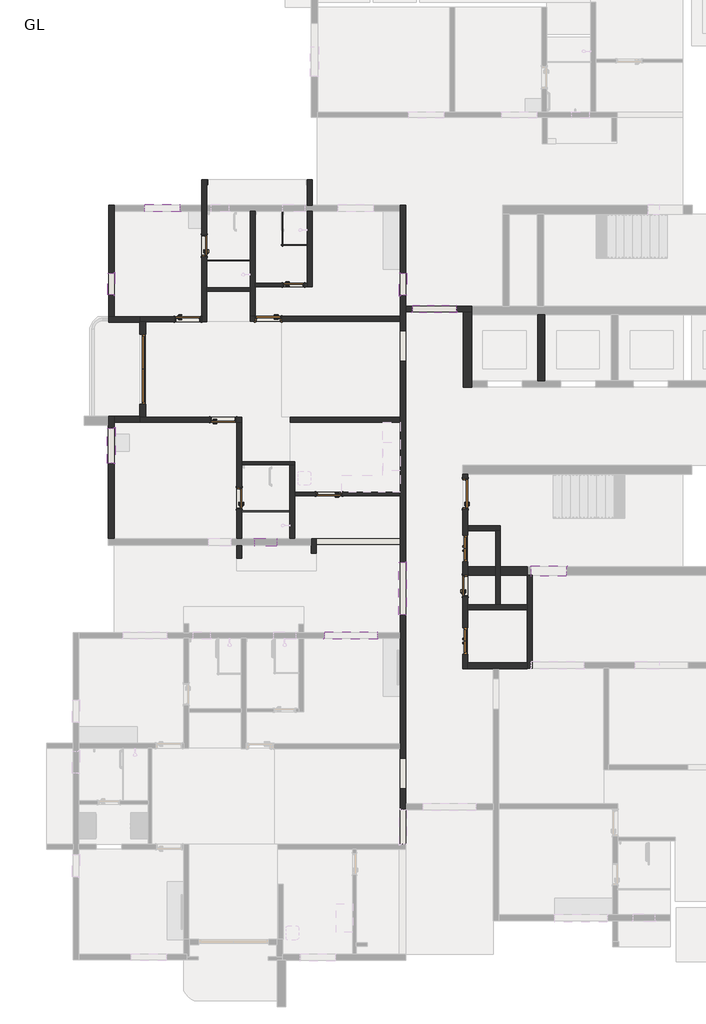
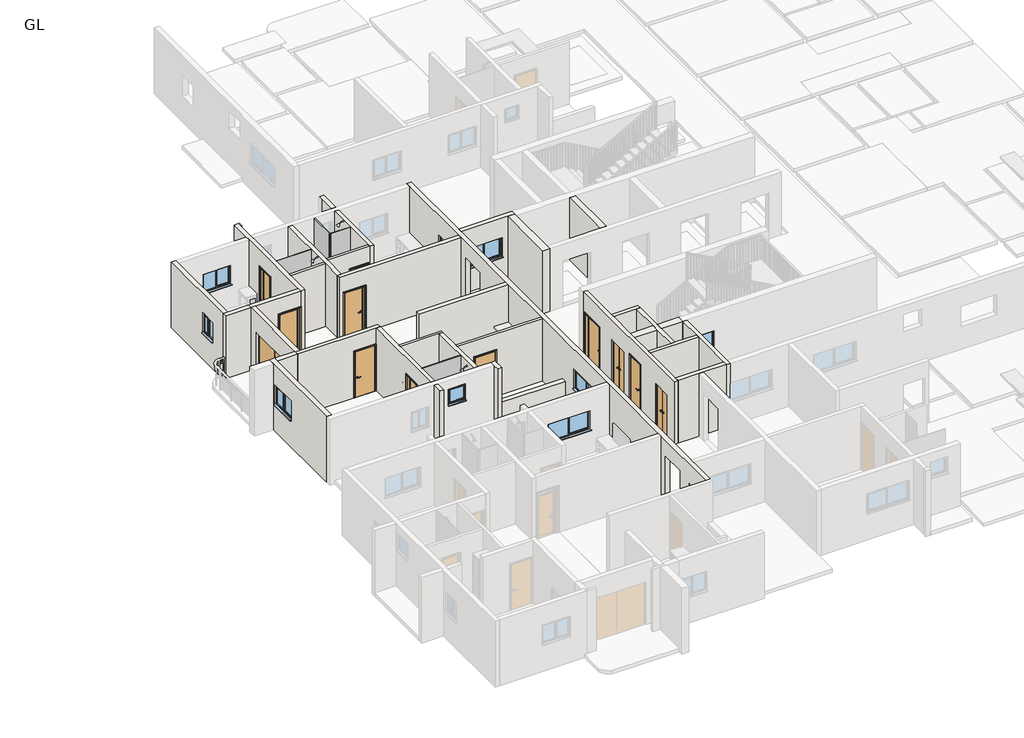
# One storey, part 2 of 14: 32 walls, 12 doors, 9 windows, 4 plates.
# Revit data of these elements (continued)
# Type "Windows_Dbl_Plain : 2.5'" (continued)
#   Analytic Construction = "1/8 in Pilkington single glazing"
#   Wrap Layers (Ext) from Ext = 0.336286 ft
#   Wrap Layers (Int) from Ext = 0.582349 ft
#   Window Board Projection = 0.082021 ft
#   Window Board Extension = 0.082021 ft
#   Visual Light Transmittance = 0.9
#   Solar Heat Gain Coefficient = 0.78
#   Rough Width = 2.5 ft
#   Rough Height = 2.985564 ft
#   Height = 2.985564 ft
#   Width = 2.5 ft
#   Heat Transfer Coefficient (U) = 3.6886 W/(m²·K)
#   Glazing Thickness = 0.07874 ft
#   FrameOffset - External = 0.164042 ft
#   Frame Depth = 0.213255 ft
#   Default Head Height = 6.922572 ft
#   Cill Depth = 0.287073 ft
#   Cavity Closer Width = 0.164042 ft
#   Cavity Closer Offset from Ext = 0.336286 ft
#   Cavity Closer Depth = 0.278871 ft
#   Vis - Cavity Closers = yes
#   Define Thermal Properties by = 1
#   Material Trim = Window Frame
#   Material Glass = Glass
#   Material Frame = Window Frame
#   Wall Closure = (empty or 0)
# Type "Windows_Dbl_Plain : 4'"
#   Type Mark = "56"
#   Operation = "DoublePanelVertical"
#   Construction Type Id = "GSP4R"
#   Manufacturer = "Revit"
#   Keynote = "L10"
#   Analytic Construction = "1/8 in Pilkington single glazing"
#   Wrap Layers (Ext) from Ext = 0.336286 ft
#   Wrap Layers (Int) from Ext = 0.582349 ft
#   Window Board Projection = 0.082021 ft
#   Window Board Extension = 0.082021 ft
#   Visual Light Transmittance = 0.9
#   Solar Heat Gain Coefficient = 0.78
#   Rough Width = 4.0 ft
#   Rough Height = 2.985564 ft
#   Height = 2.985564 ft
#   Width = 4.0 ft
#   Heat Transfer Coefficient (U) = 3.6886 W/(m²·K)
#   Glazing Thickness = 0.07874 ft
#   FrameOffset - External = 0.164042 ft
#   Frame Depth = 0.213255 ft
#   Default Head Height = 6.922572 ft
#   Cill Depth = 0.287073 ft
#   Cavity Closer Width = 0.164042 ft
#   Cavity Closer Offset from Ext = 0.336286 ft
#   Cavity Closer Depth = 0.278871 ft
#   Vis - Cavity Closers = yes
#   Define Thermal Properties by = 1
#   Material Trim = Window Frame
#   Material Glass = Glass
#   Material Frame = Window Frame
#   Wall Closure = (empty or 0)
# Type "Windows_Dbl_Plain : 5'"
#   Type Mark = "58"
#   Operation = "DoublePanelVertical"
#   Construction Type Id = "GSP4R"
#   Manufacturer = "Revit"
#   Keynote = "L10"
#   Analytic Construction = "1/8 in Pilkington single glazing"
#   Wrap Layers (Ext) from Ext = 0.336286 ft
#   Wrap Layers (Int) from Ext = 0.582349 ft
#   Window Board Projection = 0.082021 ft
#   Window Board Extension = 0.082021 ft
#   Visual Light Transmittance = 0.9
#   Solar Heat Gain Coefficient = 0.78
#   Rough Width = 5.0 ft
#   Rough Height = 2.985564 ft
#   Height = 2.985564 ft
#   Width = 5.0 ft
#   Heat Transfer Coefficient (U) = 3.6886 W/(m²·K)
#   Glazing Thickness = 0.07874 ft
#   FrameOffset - External = 0.164042 ft
#   Frame Depth = 0.213255 ft
#   Default Head Height = 6.922572 ft
#   Cill Depth = 0.287073 ft
#   Cavity Closer Width = 0.164042 ft
#   Cavity Closer Offset from Ext = 0.336286 ft
#   Cavity Closer Depth = 0.278871 ft
#   Vis - Cavity Closers = yes
#   Define Thermal Properties by = 1
#   Material Trim = Window Frame
#   Material Glass = Glass
#   Material Frame = Window Frame
#   Wall Closure = (empty or 0)
# Type "Windows_Dbl_Plain : 6'"
#   Type Mark = "62"
#   Operation = "DoublePanelVertical"
#   Construction Type Id = "GSP4R"
#   Manufacturer = "Revit"
#   Keynote = "L10"
#   Analytic Construction = "1/8 in Pilkington single glazing"
#   Wrap Layers (Ext) from Ext = 0.336286 ft
#   Wrap Layers (Int) from Ext = 0.582349 ft
#   Window Board Projection = 0.082021 ft
#   Window Board Extension = 0.082021 ft
#   Visual Light Transmittance = 0.9
#   Solar Heat Gain Coefficient = 0.78
#   Rough Width = 6.0 ft
#   Rough Height = 2.985564 ft
#   Height = 2.985564 ft
#   Width = 6.0 ft
#   Heat Transfer Coefficient (U) = 3.6886 W/(m²·K)
#   Glazing Thickness = 0.07874 ft
#   FrameOffset - External = 0.164042 ft
#   Frame Depth = 0.213255 ft
#   Default Head Height = 6.922572 ft
#   Cill Depth = 0.287073 ft
#   Cavity Closer Width = 0.164042 ft
#   Cavity Closer Offset from Ext = 0.336286 ft
#   Cavity Closer Depth = 0.278871 ft
#   Vis - Cavity Closers = yes
#   Define Thermal Properties by = 1
#   Material Trim = Window Frame
#   Material Glass = Glass
#   Material Frame = Window Frame
#   Wall Closure = (empty or 0)
# Type "Windows_Sgl_Plain : 2.5'"
#   Type Mark = "61"
#   Operation = "SinglePanel"
#   Construction Type Id = "SGL"
#   Manufacturer = "Revit"
#   Keynote = "L10"
#   Analytic Construction = "Large single-glazed windows"
#   Wrap Layers (Ext) from Ext = 0.336286 ft
#   Wrap Layers (Int) from Ext = 0.582349 ft
#   Window Board Projection = 0.082021 ft
#   Window Board Extension = 0.082021 ft
#   Visual Light Transmittance = 0.9
#   Solar Heat Gain Coefficient = 0.86
#   Rough Width = 2.5 ft
#   Rough Height = 2.5 ft
#   Height = 2.5 ft
#   Width = 2.5 ft
#   Heat Transfer Coefficient (U) = 5.5617 W/(m²·K)
#   Glazing Thickness = 0.07874 ft
#   FrameOffset - External = 0.164042 ft
#   Frame Depth = 0.213255 ft
#   Default Head Height = 6.922572 ft
#   Cill Depth = 0.287073 ft
#   Cavity Closer Width = 0.164042 ft
#   Cavity Closer Offset from Ext = 0.336286 ft
#   Cavity Closer Depth = 0.278871 ft
#   Vis - Cavity Closers = yes
#   Define Thermal Properties by = 1
#   Material Trim = Window Frame
#   Material Glass = Glass
#   Material Frame = Window Frame
#   Wall Closure = (empty or 0)
# Element 1 (IfcDoor, "Doors_Concept_ExtDbl : 8'")
#   Phase Created = New Construction
#   Materials on its faces: "Concept", "Door - Glazing"
# Elements 2, 3 (IfcDoor, "Doors_ExtDbl_Flush : 3'")
#   Phase Created = New Construction
#   Materials on its faces: "Door - Handle", "Door - Frame/Mullion", "Door - Panel"
# Elements 4, 5, 6, 7 (IfcDoor, "Doors_IntSgl : 2.5' DOOR")
#   Phase Created = New Construction
#   Materials on its faces: "Door - Architrave", "Door - Handle", "Door - Frame/Mullion (1)", "Door - Panel"
# Elements 8, 9, 10, 11 (IfcDoor, "Doors_IntSgl : 3' DOOR")
#   Phase Created = New Construction
#   Materials on its faces: "Door - Architrave", "Door - Handle", "Door - Frame/Mullion (1)", "Door - Panel"
# Element 12 (IfcDoor, "Doors_IntSgl : 3.5'")
#   Phase Created = New Construction
#   Materials on its faces: "Door - Architrave", "Door - Handle", "Door - Frame/Mullion (1)", "Door - Panel"
# Elements 13, 14, 15, 16 (IfcPlate, "System Panel : Glazed")
#   Phase Created = New Construction
#   Materials on its faces: "Glass"
# Elements 17, 18, 19, 20, 21, 22, 23, 24, 25 (IfcWall, "W2")
#   Top Offset = 0.0 ft
#   Base Offset = 0.0 ft
#   wall height = 9.84252 ft
#   Phase Created = New Construction
#   Base Constraint = GL
#   Top Constraint = FFL
#   Materials on its faces: "Brick, Common"
# Elements 26, 27, 28, 29 (IfcWall, "W3")
#   Top Offset = 0.0 ft
#   Base Offset = 0.0 ft
#   wall height = 9.84252 ft
#   Phase Created = New Construction
#   Base Constraint = GL
#   Top Constraint = FFL
#   Materials on its faces: "Brick, Common"
# Elements 30, 31 (IfcWall, "W4")
#   Top Offset = 0.0 ft
#   Base Offset = 0.0 ft
#   wall height = 9.84252 ft
#   Phase Created = New Construction
#   Base Constraint = GL
#   Top Constraint = FFL
#   Materials on its faces: "Brick, Common"
# Element 32 (IfcWall, "W6")
#   Top Offset = 0.0 ft
#   Base Offset = 0.0 ft
#   wall height = 9.84252 ft
#   Phase Created = New Construction
#   Base Constraint = GL
#   Top Constraint = FFL
#   Materials on its faces: "Brick, Common"
# Element 33 (IfcWall, "W8")
#   Top Offset = 0.0 ft
#   Base Offset = 0.0 ft
#   wall height = 9.84252 ft
#   Phase Created = New Construction
#   Base Constraint = GL
#   Top Constraint = FFL
#   Materials on its faces: "Brick, Common"
# Elements 34, 35, 36, 37, 38, 39, 40 (IfcWall, "W9")
#   Top Offset = 0.0 ft
#   Base Offset = 0.0 ft
#   wall height = 9.84252 ft
#   Phase Created = New Construction
#   Base Constraint = GL
#   Top Constraint = FFL
#   Materials on its faces: "Brick, Common"
# Elements 41, 42, 44, 45, 46, 47, 48 (IfcWall, "WALL 1")
#   Top Offset = 0.0 ft
#   Base Offset = 0.0 ft
#   wall height = 9.84252 ft
#   Phase Created = New Construction
#   Base Constraint = GL
#   Top Constraint = FFL
#   Materials on its faces: "Brick, Common"
# Element 43 (IfcWall, "WALL 1")
#   Top Offset = -6.0 ft
#   Base Offset = 0.0 ft
#   wall height = 3.84252 ft
#   Phase Created = New Construction
#   Base Constraint = GL
#   Top Constraint = FFL
#   Materials on its faces: "Brick, Common"
# Element 49 (IfcWindow, "Windows_Dbl_Plain : 2.5'")
#   Mark = "62"
#   Phase Created = New Construction
#   Materials on its faces: "Window Frame", "Glass"
# Element 50 (IfcWindow, "Windows_Dbl_Plain : 2.5'")
#   Mark = "67"
#   Phase Created = New Construction
#   Materials on its faces: "Window Frame", "Glass"
# Element 51 (IfcWindow, "Windows_Dbl_Plain : 4'")
#   Mark = "63"
#   Phase Created = New Construction
#   Materials on its faces: "Window Frame", "Glass"
# Element 52 (IfcWindow, "Windows_Dbl_Plain : 4'")
#   Mark = "60"
#   Phase Created = New Construction
#   Materials on its faces: "Window Frame", "Glass"
# Element 53 (IfcWindow, "Windows_Dbl_Plain : 4'")
#   Mark = "25"
#   Phase Created = New Construction
#   Materials on its faces: "Window Frame", "Glass"
# Element 54 (IfcWindow, "Windows_Dbl_Plain : 5'")
#   Mark = "68"
#   Phase Created = New Construction
#   Materials on its faces: "Window Frame", "Glass"
# Element 55 (IfcWindow, "Windows_Dbl_Plain : 6'")
#   Mark = "9"
#   Phase Created = New Construction
#   Materials on its faces: "Window Frame", "Glass"
# Element 56 (IfcWindow, "Windows_Dbl_Plain : 6'")
#   Mark = "24"
#   Phase Created = New Construction
#   Materials on its faces: "Window Frame", "Glass"
# Element 57 (IfcWindow, "Windows_Sgl_Plain : 2.5'")
#   Mark = "58"
#   Phase Created = New Construction
#   Materials on its faces: "Window Frame", "Glass"
# Materials
#   "Door - Glazing": colour RGB 0 0 255, transparency 0.75
#   "Concept": colour RGB 128 128 255, transparency 0.5
#   "Door - Panel": class "Wood", colour RGB 210 159 95, transparency 0, Keynote = "L20", Cost = 0
#   "Door - Frame/Mullion": class "Wood", colour RGB 212 179 113, transparency 0, Keynote = "L20", Cost = 0
#   "Door - Handle": colour RGB 0 0 0, transparency 0, Keynote = "P21", Cost = 0
#   "Door - Frame/Mullion (1)": class "Wood", colour RGB 212 179 113, transparency 0, Keynote = "L20", Cost = 0
#   "Door - Architrave": class "Wood", colour RGB 154 90 5, transparency 0, Keynote = "P20", Cost = 0
#   "Brick, Common": class "Masonry", colour RGB 170 100 105, transparency 0, Description = "Common brick", Cost = 0
#   "Window Frame": colour RGB 249 249 249, transparency 0, Keynote = "L10", Cost = 0
#   "Glass": class "Glass", colour RGB 0 128 192, transparency 0.9, Description = "Soda Lime Glass", Cost = 0
